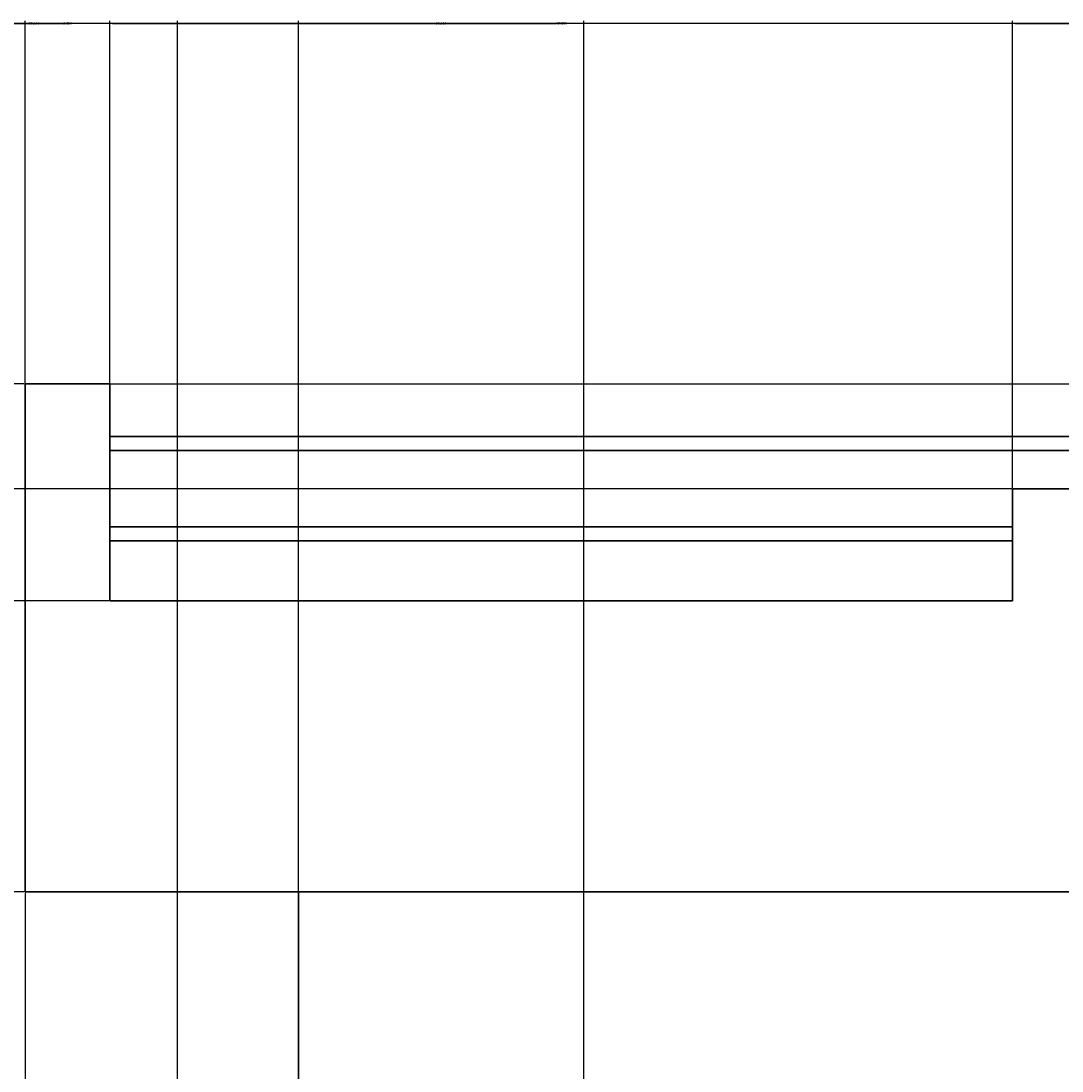
# Model space of a CAD drawing. Units: inches. Extents: x 93 to 565, y 123 to 656.
# Tile 17 of 18: x 418 to 491, y 582 to 656. Entities that reach past the tile are written whole.
import ezdxf

# ---------------------------------------------------------------- set-up
doc = ezdxf.new("R2010")
doc.units = ezdxf.units.IN
doc.header["$MEASUREMENT"] = 0
doc.layers.add('A-ANNO-DIMS', color=2, linetype='Continuous', lineweight=18)
doc.layers.add('A-ELEV', color=7, linetype='Continuous', lineweight=35)
doc.styles.get("Standard").update_dxf_attribs({"font": 'arial.ttf'})
doc.dimstyles.get("Standard").update_dxf_attribs({"dimtxt": 0.18, "dimasz": 0.18, "dimexe": 0.18, "dimexo": 0.0625, "dimgap": 0.09, "dimtad": 0, "dimtih": 1, "dimtoh": 1, "dimdec": 4, "dimzin": 0, "dimdsep": 46, "dimtxsty": 'Standard', "dimcen": 0.09, "dimadec": 0, "dimazin": 0, "dimtfac": 1, "dimtdec": 4, "dimtofl": 0, "dimtmove": 0, "dimatfit": 3, "dimfxl": 1, "dimtolj": 1, "dimtzin": 0, "dimarcsym": 0})

# ---------------------------------------------------------------- blocks, each defined once
blk = doc.blocks.new('*D26')
at = {"layer": 'A-ANNO-DIMS', "color": 0, "lineweight": -2, "transparency": 16777216}
for p, q in [((119.079, 519.162), (119.079, 656.135)), ((119.259, 655.955), (328.787, 655.955)), ((538.899, 655.955), (329.372, 655.955)), ((539.079, 630.467), (539.079, 656.135))]:
    blk.add_line(p, q, dxfattribs=at)
at = {"layer": 'A-ANNO-DIMS', "color": 0, "transparency": 16777216}
for points in [[(119.259, 655.985), (119.259, 655.925), (119.079, 655.955)], [(538.899, 655.985), (538.899, 655.925), (539.079, 655.955)]]:
    blk.add_solid(points, dxfattribs=at)
at = {"layer": 'Defpoints', "color": 0, "transparency": 16777216}
for p in [(539.079, 655.955), (539.079, 630.405), (119.079, 519.1)]:
    blk.add_point(p, dxfattribs=at)
at = {"layer": 'A-ANNO-DIMS', "color": 0, "transparency": 16777216, "insert": (329.079, 655.955), "char_height": 0.18, "attachment_point": 5}
blk.add_mtext('\\A1;420', dxfattribs=at)
blk = doc.blocks.new('*D29')
at = {"layer": 'A-ANNO-DIMS', "color": 0, "lineweight": -2, "transparency": 16777216}
for p, q in [((437.189, 594.342), (437.189, 134.002)), ((295.687, 183.67), (295.687, 134.002)), ((295.867, 134.182), (366.052, 134.182)), ((437.009, 134.182), (366.824, 134.182))]:
    blk.add_line(p, q, dxfattribs=at)
at = {"layer": 'A-ANNO-DIMS', "color": 0, "transparency": 16777216}
for points in [[(295.867, 134.212), (295.867, 134.152), (295.687, 134.182)], [(437.009, 134.212), (437.009, 134.152), (437.189, 134.182)]]:
    blk.add_solid(points, dxfattribs=at)
at = {"layer": 'Defpoints', "color": 0, "transparency": 16777216}
for p in [(437.189, 594.405), (295.687, 183.732), (437.189, 134.182)]:
    blk.add_point(p, dxfattribs=at)
at = {"layer": 'A-ANNO-DIMS', "color": 0, "transparency": 16777216, "insert": (366.438, 134.182), "char_height": 0.18, "attachment_point": 5}
blk.add_mtext('\\A1;141.5', dxfattribs=at)
blk = doc.blocks.new('*D30')
at = {"layer": 'A-ANNO-DIMS', "color": 0, "lineweight": -2, "transparency": 16777216}
for p, q in [((437.189, 594.342), (437.189, 134.002)), ((539.079, 159.67), (539.079, 134.002)), ((437.369, 134.182), (487.749, 134.182)), ((538.899, 134.182), (488.519, 134.182))]:
    blk.add_line(p, q, dxfattribs=at)
at = {"layer": 'A-ANNO-DIMS', "color": 0, "transparency": 16777216}
for points in [[(437.369, 134.212), (437.369, 134.152), (437.189, 134.182)], [(538.899, 134.212), (538.899, 134.152), (539.079, 134.182)]]:
    blk.add_solid(points, dxfattribs=at)
at = {"layer": 'Defpoints', "color": 0, "transparency": 16777216}
for p in [(437.189, 594.405), (539.079, 159.732), (539.079, 134.182)]:
    blk.add_point(p, dxfattribs=at)
at = {"layer": 'A-ANNO-DIMS', "color": 0, "transparency": 16777216, "insert": (488.134, 134.182), "char_height": 0.18, "attachment_point": 5}
blk.add_mtext('\\A1;101.9', dxfattribs=at)
blk = doc.blocks.new('*D31')
at = {"layer": 'A-ANNO-DIMS', "color": 0, "lineweight": -2, "transparency": 16777216}
for p, q in [((417.872, 630.405), (564.809, 630.405)), ((564.629, 630.225), (564.629, 395.25)), ((564.629, 159.912), (564.629, 394.887)), ((119.142, 159.732), (564.809, 159.732))]:
    blk.add_line(p, q, dxfattribs=at)
at = {"layer": 'A-ANNO-DIMS', "color": 0, "transparency": 16777216}
for points in [[(564.599, 630.225), (564.659, 630.225), (564.629, 630.405)], [(564.599, 159.912), (564.659, 159.912), (564.629, 159.732)]]:
    blk.add_solid(points, dxfattribs=at)
at = {"layer": 'Defpoints', "color": 0, "transparency": 16777216}
for p in [(417.81, 630.405), (564.629, 630.405), (119.079, 159.732)]:
    blk.add_point(p, dxfattribs=at)
at = {"layer": 'A-ANNO-DIMS', "color": 0, "transparency": 16777216, "insert": (564.629, 395.069), "char_height": 0.18, "attachment_point": 5}
blk.add_mtext('\\A1;470.7', dxfattribs=at)
blk = doc.blocks.new('*D36')
at = {"layer": 'A-ANNO-DIMS', "color": 0, "lineweight": -2, "transparency": 16777216}
for p, q in [((417.747, 594.405), (93.349, 594.405)), ((93.529, 594.225), (93.529, 556.934)), ((93.529, 519.28), (93.529, 556.57)), ((119.017, 519.1), (93.349, 519.1))]:
    blk.add_line(p, q, dxfattribs=at)
at = {"layer": 'A-ANNO-DIMS', "color": 0, "transparency": 16777216}
for points in [[(93.499, 594.225), (93.559, 594.225), (93.529, 594.405)], [(93.499, 519.28), (93.559, 519.28), (93.529, 519.1)]]:
    blk.add_solid(points, dxfattribs=at)
at = {"layer": 'Defpoints', "color": 0, "transparency": 16777216}
for p in [(93.529, 594.405), (417.81, 594.405), (119.079, 519.1)]:
    blk.add_point(p, dxfattribs=at)
at = {"layer": 'A-ANNO-DIMS', "color": 0, "transparency": 16777216, "insert": (93.529, 556.752), "char_height": 0.18, "attachment_point": 5}
blk.add_mtext('\\A1;75.3', dxfattribs=at)
blk = doc.blocks.new('*D69')
at = {"layer": 'A-ANNO-DIMS', "color": 0, "lineweight": -2, "transparency": 16777216}
for p, q in [((355.46, 420.63), (355.46, 656.135)), ((355.64, 655.955), (391.645, 655.955)), ((428.436, 655.955), (392.431, 655.955)), ((428.616, 420.63), (428.616, 656.135))]:
    blk.add_line(p, q, dxfattribs=at)
at = {"layer": 'A-ANNO-DIMS', "color": 0, "transparency": 16777216}
for points in [[(355.64, 655.985), (355.64, 655.925), (355.46, 655.955)], [(428.436, 655.985), (428.436, 655.925), (428.616, 655.955)]]:
    blk.add_solid(points, dxfattribs=at)
at = {"layer": 'Defpoints', "color": 0, "transparency": 16777216}
for p in [(428.616, 655.955), (355.46, 420.567), (428.616, 420.567)]:
    blk.add_point(p, dxfattribs=at)
at = {"layer": 'A-ANNO-DIMS', "color": 0, "transparency": 16777216, "insert": (392.038, 655.955), "char_height": 0.18, "attachment_point": 5}
blk.add_mtext('\\A1;73.16', dxfattribs=at)
blk = doc.blocks.new('*D76')
at = {"layer": 'A-ANNO-DIMS', "color": 0, "lineweight": -2, "transparency": 16777216}
for p, q in [((399.695, 507.892), (399.695, 656.135)), ((399.875, 655.955), (417.978, 655.955)), ((437.009, 655.955), (418.905, 655.955)), ((437.189, 507.795), (437.189, 656.135))]:
    blk.add_line(p, q, dxfattribs=at)
at = {"layer": 'A-ANNO-DIMS', "color": 0, "transparency": 16777216}
for points in [[(399.875, 655.985), (399.875, 655.925), (399.695, 655.955)], [(437.009, 655.985), (437.009, 655.925), (437.189, 655.955)]]:
    blk.add_solid(points, dxfattribs=at)
at = {"layer": 'Defpoints', "color": 0, "transparency": 16777216}
for p in [(437.189, 655.955), (399.695, 507.83), (437.189, 507.732)]:
    blk.add_point(p, dxfattribs=at)
at = {"layer": 'A-ANNO-DIMS', "color": 0, "transparency": 16777216, "insert": (418.442, 655.955), "char_height": 0.18, "attachment_point": 5}
blk.add_mtext('\\A1;37.494', dxfattribs=at)
blk = doc.blocks.new('*D82')
at = {"layer": 'A-ANNO-DIMS', "color": 0, "lineweight": -2, "transparency": 16777216}
for p, q in [((437.189, 447.795), (437.189, 656.135)), ((437.369, 655.955), (446.825, 655.955)), ((457.213, 655.955), (447.757, 655.955)), ((457.393, 378.4), (457.393, 656.135))]:
    blk.add_line(p, q, dxfattribs=at)
at = {"layer": 'A-ANNO-DIMS', "color": 0, "transparency": 16777216}
for points in [[(437.369, 655.985), (437.369, 655.925), (437.189, 655.955)], [(457.213, 655.985), (457.213, 655.925), (457.393, 655.955)]]:
    blk.add_solid(points, dxfattribs=at)
at = {"layer": 'Defpoints', "color": 0, "transparency": 16777216}
for p in [(457.393, 655.955), (437.189, 447.732), (457.393, 378.337)]:
    blk.add_point(p, dxfattribs=at)
at = {"layer": 'A-ANNO-DIMS', "color": 0, "transparency": 16777216, "insert": (447.291, 655.955), "char_height": 0.18, "attachment_point": 5}
blk.add_mtext('\\A1;20.205', dxfattribs=at)
blk = doc.blocks.new('*D86')
at = {"layer": 'A-ANNO-DIMS', "color": 0, "lineweight": -2, "transparency": 16777216}
for p, q in [((417.81, 630.467), (417.81, 656.135)), ((417.99, 655.955), (420.66, 655.955)), ((423.63, 655.955), (420.959, 655.955)), ((423.81, 630.467), (423.81, 656.135))]:
    blk.add_line(p, q, dxfattribs=at)
at = {"layer": 'A-ANNO-DIMS', "color": 0, "transparency": 16777216}
for points in [[(417.99, 655.985), (417.99, 655.925), (417.81, 655.955)], [(423.63, 655.985), (423.63, 655.925), (423.81, 655.955)]]:
    blk.add_solid(points, dxfattribs=at)
at = {"layer": 'Defpoints', "color": 0, "transparency": 16777216}
for p in [(423.81, 655.955), (417.81, 630.405), (423.81, 630.405)]:
    blk.add_point(p, dxfattribs=at)
at = {"layer": 'A-ANNO-DIMS', "color": 0, "transparency": 16777216, "insert": (420.81, 655.955), "char_height": 0.18, "attachment_point": 5}
blk.add_mtext('\\A1;6', dxfattribs=at)
blk = doc.blocks.new('*D87')
at = {"layer": 'A-ANNO-DIMS', "color": 0, "lineweight": -2, "transparency": 16777216}
for p, q in [((423.81, 630.467), (423.81, 656.135)), ((423.99, 655.955), (455.408, 655.955)), ((487.615, 655.955), (456.197, 655.955)), ((487.795, 623.034), (487.795, 656.135))]:
    blk.add_line(p, q, dxfattribs=at)
at = {"layer": 'A-ANNO-DIMS', "color": 0, "transparency": 16777216}
for points in [[(423.99, 655.985), (423.99, 655.925), (423.81, 655.955)], [(487.615, 655.985), (487.615, 655.925), (487.795, 655.955)]]:
    blk.add_solid(points, dxfattribs=at)
at = {"layer": 'Defpoints', "color": 0, "transparency": 16777216}
for p in [(487.795, 655.955), (423.81, 630.405), (487.795, 622.971)]:
    blk.add_point(p, dxfattribs=at)
at = {"layer": 'A-ANNO-DIMS', "color": 0, "transparency": 16777216, "insert": (455.802, 655.955), "char_height": 0.18, "attachment_point": 5}
blk.add_mtext('\\A1;63.99', dxfattribs=at)
blk = doc.blocks.new('*D88')
at = {"layer": 'A-ANNO-DIMS', "color": 0, "lineweight": -2, "transparency": 16777216}
for p, q in [((487.795, 623.034), (487.795, 656.135)), ((487.975, 655.955), (500.917, 655.955)), ((514.789, 655.955), (501.847, 655.955)), ((514.969, 630.467), (514.969, 656.135))]:
    blk.add_line(p, q, dxfattribs=at)
at = {"layer": 'A-ANNO-DIMS', "color": 0, "transparency": 16777216}
for points in [[(487.975, 655.985), (487.975, 655.925), (487.795, 655.955)], [(514.789, 655.985), (514.789, 655.925), (514.969, 655.955)]]:
    blk.add_solid(points, dxfattribs=at)
at = {"layer": 'Defpoints', "color": 0, "transparency": 16777216}
for p in [(514.969, 655.955), (514.969, 630.405), (487.795, 622.971)]:
    blk.add_point(p, dxfattribs=at)
at = {"layer": 'A-ANNO-DIMS', "color": 0, "transparency": 16777216, "insert": (501.382, 655.955), "char_height": 0.18, "attachment_point": 5}
blk.add_mtext('\\A1;27.174', dxfattribs=at)
blk = doc.blocks.new('*D90')
at = {"layer": 'A-ANNO-DIMS', "color": 0, "lineweight": -2, "transparency": 16777216}
for p, q in [((417.81, 594.342), (417.81, 134.002)), ((437.189, 594.342), (437.189, 134.002)), ((417.99, 134.182), (427.114, 134.182)), ((437.009, 134.182), (427.885, 134.182))]:
    blk.add_line(p, q, dxfattribs=at)
at = {"layer": 'A-ANNO-DIMS', "color": 0, "transparency": 16777216}
for points in [[(417.99, 134.212), (417.99, 134.152), (417.81, 134.182)], [(437.009, 134.212), (437.009, 134.152), (437.189, 134.182)]]:
    blk.add_solid(points, dxfattribs=at)
at = {"layer": 'Defpoints', "color": 0, "transparency": 16777216}
for p in [(417.81, 594.405), (437.189, 594.405), (437.189, 134.182)]:
    blk.add_point(p, dxfattribs=at)
at = {"layer": 'A-ANNO-DIMS', "color": 0, "transparency": 16777216, "insert": (427.499, 134.182), "char_height": 0.18, "attachment_point": 5}
blk.add_mtext('\\A1;19.38', dxfattribs=at)
blk = doc.blocks.new('*D91')
at = {"layer": 'A-ANNO-DIMS', "color": 0, "lineweight": -2, "transparency": 16777216}
for p, q in [((499.729, 599.755), (499.729, 134.002)), ((437.189, 594.342), (437.189, 134.002)), ((437.369, 134.182), (468.065, 134.182)), ((499.549, 134.182), (468.853, 134.182))]:
    blk.add_line(p, q, dxfattribs=at)
at = {"layer": 'A-ANNO-DIMS', "color": 0, "transparency": 16777216}
for points in [[(437.369, 134.212), (437.369, 134.152), (437.189, 134.182)], [(499.549, 134.212), (499.549, 134.152), (499.729, 134.182)]]:
    blk.add_solid(points, dxfattribs=at)
at = {"layer": 'Defpoints', "color": 0, "transparency": 16777216}
for p in [(499.729, 599.817), (437.189, 594.405), (499.729, 134.182)]:
    blk.add_point(p, dxfattribs=at)
at = {"layer": 'A-ANNO-DIMS', "color": 0, "transparency": 16777216, "insert": (468.459, 134.182), "char_height": 0.18, "attachment_point": 5}
blk.add_mtext('\\A1;62.54', dxfattribs=at)
blk = doc.blocks.new('*D94')
at = {"layer": 'A-ANNO-DIMS', "color": 0, "lineweight": -2, "transparency": 16777216}
for p, q in [((423.747, 615.041), (93.349, 615.041)), ((93.529, 614.861), (93.529, 604.905)), ((93.529, 594.585), (93.529, 604.541)), ((417.747, 594.405), (93.349, 594.405))]:
    blk.add_line(p, q, dxfattribs=at)
at = {"layer": 'A-ANNO-DIMS', "color": 0, "transparency": 16777216}
for points in [[(93.499, 614.861), (93.559, 614.861), (93.529, 615.041)], [(93.499, 594.585), (93.559, 594.585), (93.529, 594.405)]]:
    blk.add_solid(points, dxfattribs=at)
at = {"layer": 'Defpoints', "color": 0, "transparency": 16777216}
for p in [(93.529, 615.041), (423.81, 615.041), (417.81, 594.405)]:
    blk.add_point(p, dxfattribs=at)
at = {"layer": 'A-ANNO-DIMS', "color": 0, "transparency": 16777216, "insert": (93.529, 604.723), "char_height": 0.18, "attachment_point": 5}
blk.add_mtext('\\A1;20.636', dxfattribs=at)
blk = doc.blocks.new('*D95')
at = {"layer": 'A-ANNO-DIMS', "color": 0, "lineweight": -2, "transparency": 16777216}
for p, q in [((487.733, 622.971), (93.349, 622.971)), ((93.529, 622.791), (93.529, 619.188)), ((93.529, 615.221), (93.529, 618.824)), ((423.747, 615.041), (93.349, 615.041))]:
    blk.add_line(p, q, dxfattribs=at)
at = {"layer": 'A-ANNO-DIMS', "color": 0, "transparency": 16777216}
for points in [[(93.499, 622.791), (93.559, 622.791), (93.529, 622.971)], [(93.499, 615.221), (93.559, 615.221), (93.529, 615.041)]]:
    blk.add_solid(points, dxfattribs=at)
at = {"layer": 'Defpoints', "color": 0, "transparency": 16777216}
for p in [(93.529, 622.971), (487.795, 622.971), (423.81, 615.041)]:
    blk.add_point(p, dxfattribs=at)
at = {"layer": 'A-ANNO-DIMS', "color": 0, "transparency": 16777216, "insert": (93.529, 619.006), "char_height": 0.18, "attachment_point": 5}
blk.add_mtext('\\A1;7.93', dxfattribs=at)
blk = doc.blocks.new('*D96')
at = {"layer": 'A-ANNO-DIMS', "color": 0, "lineweight": -2, "transparency": 16777216}
for p, q in [((417.747, 630.405), (93.349, 630.405)), ((93.529, 630.225), (93.529, 626.87)), ((93.529, 623.151), (93.529, 626.506)), ((487.733, 622.971), (93.349, 622.971))]:
    blk.add_line(p, q, dxfattribs=at)
at = {"layer": 'A-ANNO-DIMS', "color": 0, "transparency": 16777216}
for points in [[(93.499, 630.225), (93.559, 630.225), (93.529, 630.405)], [(93.499, 623.151), (93.559, 623.151), (93.529, 622.971)]]:
    blk.add_solid(points, dxfattribs=at)
at = {"layer": 'Defpoints', "color": 0, "transparency": 16777216}
for p in [(93.529, 630.405), (417.81, 630.405), (487.795, 622.971)]:
    blk.add_point(p, dxfattribs=at)
at = {"layer": 'A-ANNO-DIMS', "color": 0, "transparency": 16777216, "insert": (93.529, 626.688), "char_height": 0.18, "attachment_point": 5}
blk.add_mtext('\\A1;7.434', dxfattribs=at)
blk = doc.blocks.new('*D100')
at = {"layer": 'A-ANNO-DIMS', "color": 0, "lineweight": -2, "transparency": 16777216}
for p, q in [((499.792, 599.817), (564.809, 599.817)), ((564.629, 599.637), (564.629, 597.293)), ((564.629, 594.585), (564.629, 596.929)), ((437.251, 594.405), (564.809, 594.405))]:
    blk.add_line(p, q, dxfattribs=at)
at = {"layer": 'A-ANNO-DIMS', "color": 0, "transparency": 16777216}
for points in [[(564.599, 599.637), (564.659, 599.637), (564.629, 599.817)], [(564.599, 594.585), (564.659, 594.585), (564.629, 594.405)]]:
    blk.add_solid(points, dxfattribs=at)
at = {"layer": 'Defpoints', "color": 0, "transparency": 16777216}
for p in [(499.729, 599.817), (437.189, 594.405), (564.629, 594.405)]:
    blk.add_point(p, dxfattribs=at)
at = {"layer": 'A-ANNO-DIMS', "color": 0, "transparency": 16777216, "insert": (564.629, 597.111), "char_height": 0.18, "attachment_point": 5}
blk.add_mtext('\\A1;5.412', dxfattribs=at)
blk = doc.blocks.new('*D105')
at = {"layer": 'A-ANNO-DIMS', "color": 0, "lineweight": -2, "transparency": 16777216}
for p, q in [((119.079, 519.162), (119.079, 656.135)), ((119.259, 655.955), (328.542, 655.955)), ((538.899, 655.955), (329.616, 655.955)), ((539.079, 630.467), (539.079, 656.135))]:
    blk.add_line(p, q, dxfattribs=at)
at = {"layer": 'A-ANNO-DIMS', "color": 0, "transparency": 16777216}
for points in [[(119.259, 655.985), (119.259, 655.925), (119.079, 655.955)], [(538.899, 655.985), (538.899, 655.925), (539.079, 655.955)]]:
    blk.add_solid(points, dxfattribs=at)
at = {"layer": 'Defpoints', "color": 0, "transparency": 16777216}
for p in [(539.079, 655.955), (539.079, 630.405), (119.079, 519.1)]:
    blk.add_point(p, dxfattribs=at)
at = {"layer": 'A-ANNO-DIMS', "color": 0, "transparency": 16777216, "insert": (329.079, 655.955), "char_height": 0.18, "attachment_point": 5}
blk.add_mtext('\\A1;420.000', dxfattribs=at)
blk = doc.blocks.new('*D108')
at = {"layer": 'A-ANNO-DIMS', "color": 0, "lineweight": -2, "transparency": 16777216}
for p, q in [((437.189, 594.342), (437.189, 134.002)), ((295.687, 183.67), (295.687, 134.002)), ((295.867, 134.182), (365.93, 134.182)), ((437.009, 134.182), (366.946, 134.182))]:
    blk.add_line(p, q, dxfattribs=at)
at = {"layer": 'A-ANNO-DIMS', "color": 0, "transparency": 16777216}
for points in [[(295.867, 134.212), (295.867, 134.152), (295.687, 134.182)], [(437.009, 134.212), (437.009, 134.152), (437.189, 134.182)]]:
    blk.add_solid(points, dxfattribs=at)
at = {"layer": 'Defpoints', "color": 0, "transparency": 16777216}
for p in [(437.189, 594.405), (295.687, 183.732), (437.189, 134.182)]:
    blk.add_point(p, dxfattribs=at)
at = {"layer": 'A-ANNO-DIMS', "color": 0, "transparency": 16777216, "insert": (366.438, 134.182), "char_height": 0.18, "attachment_point": 5}
blk.add_mtext('\\A1;141.501', dxfattribs=at)
blk = doc.blocks.new('*D109')
at = {"layer": 'A-ANNO-DIMS', "color": 0, "lineweight": -2, "transparency": 16777216}
for p, q in [((437.189, 594.342), (437.189, 134.002)), ((539.079, 159.67), (539.079, 134.002)), ((437.369, 134.182), (487.626, 134.182)), ((538.899, 134.182), (488.642, 134.182))]:
    blk.add_line(p, q, dxfattribs=at)
at = {"layer": 'A-ANNO-DIMS', "color": 0, "transparency": 16777216}
for points in [[(437.369, 134.212), (437.369, 134.152), (437.189, 134.182)], [(538.899, 134.212), (538.899, 134.152), (539.079, 134.182)]]:
    blk.add_solid(points, dxfattribs=at)
at = {"layer": 'Defpoints', "color": 0, "transparency": 16777216}
for p in [(437.189, 594.405), (539.079, 159.732), (539.079, 134.182)]:
    blk.add_point(p, dxfattribs=at)
at = {"layer": 'A-ANNO-DIMS', "color": 0, "transparency": 16777216, "insert": (488.134, 134.182), "char_height": 0.18, "attachment_point": 5}
blk.add_mtext('\\A1;101.891', dxfattribs=at)
blk = doc.blocks.new('*D110')
at = {"layer": 'A-ANNO-DIMS', "color": 0, "lineweight": -2, "transparency": 16777216}
for p, q in [((417.872, 630.405), (564.809, 630.405)), ((564.629, 630.225), (564.629, 395.25)), ((564.629, 159.912), (564.629, 394.887)), ((119.142, 159.732), (564.809, 159.732))]:
    blk.add_line(p, q, dxfattribs=at)
at = {"layer": 'A-ANNO-DIMS', "color": 0, "transparency": 16777216}
for points in [[(564.599, 630.225), (564.659, 630.225), (564.629, 630.405)], [(564.599, 159.912), (564.659, 159.912), (564.629, 159.732)]]:
    blk.add_solid(points, dxfattribs=at)
at = {"layer": 'Defpoints', "color": 0, "transparency": 16777216}
for p in [(417.81, 630.405), (564.629, 630.405), (119.079, 159.732)]:
    blk.add_point(p, dxfattribs=at)
at = {"layer": 'A-ANNO-DIMS', "color": 0, "transparency": 16777216, "insert": (564.629, 395.069), "char_height": 0.18, "attachment_point": 5}
blk.add_mtext('\\A1;470.673', dxfattribs=at)
blk = doc.blocks.new('*D115')
at = {"layer": 'A-ANNO-DIMS', "color": 0, "lineweight": -2, "transparency": 16777216}
for p, q in [((417.747, 594.405), (93.349, 594.405)), ((93.529, 594.225), (93.529, 556.934)), ((93.529, 519.28), (93.529, 556.57)), ((119.017, 519.1), (93.349, 519.1))]:
    blk.add_line(p, q, dxfattribs=at)
at = {"layer": 'A-ANNO-DIMS', "color": 0, "transparency": 16777216}
for points in [[(93.499, 594.225), (93.559, 594.225), (93.529, 594.405)], [(93.499, 519.28), (93.559, 519.28), (93.529, 519.1)]]:
    blk.add_solid(points, dxfattribs=at)
at = {"layer": 'Defpoints', "color": 0, "transparency": 16777216}
for p in [(93.529, 594.405), (417.81, 594.405), (119.079, 519.1)]:
    blk.add_point(p, dxfattribs=at)
at = {"layer": 'A-ANNO-DIMS', "color": 0, "transparency": 16777216, "insert": (93.529, 556.752), "char_height": 0.18, "attachment_point": 5}
blk.add_mtext('\\A1;75.305', dxfattribs=at)
blk = doc.blocks.new('*D148')
at = {"layer": 'A-ANNO-DIMS', "color": 0, "lineweight": -2, "transparency": 16777216}
for p, q in [((355.46, 420.63), (355.46, 656.135)), ((355.64, 655.955), (391.575, 655.955)), ((428.436, 655.955), (392.501, 655.955)), ((428.616, 420.63), (428.616, 656.135))]:
    blk.add_line(p, q, dxfattribs=at)
at = {"layer": 'A-ANNO-DIMS', "color": 0, "transparency": 16777216}
for points in [[(355.64, 655.985), (355.64, 655.925), (355.46, 655.955)], [(428.436, 655.985), (428.436, 655.925), (428.616, 655.955)]]:
    blk.add_solid(points, dxfattribs=at)
at = {"layer": 'Defpoints', "color": 0, "transparency": 16777216}
for p in [(428.616, 655.955), (355.46, 420.567), (428.616, 420.567)]:
    blk.add_point(p, dxfattribs=at)
at = {"layer": 'A-ANNO-DIMS', "color": 0, "transparency": 16777216, "insert": (392.038, 655.955), "char_height": 0.18, "attachment_point": 5}
blk.add_mtext('\\A1;73.156', dxfattribs=at)
blk = doc.blocks.new('*D155')
at = {"layer": 'A-ANNO-DIMS', "color": 0, "lineweight": -2, "transparency": 16777216}
for p, q in [((399.695, 507.892), (399.695, 656.135)), ((399.875, 655.955), (417.978, 655.955)), ((437.009, 655.955), (418.905, 655.955)), ((437.189, 507.795), (437.189, 656.135))]:
    blk.add_line(p, q, dxfattribs=at)
at = {"layer": 'A-ANNO-DIMS', "color": 0, "transparency": 16777216}
for points in [[(399.875, 655.985), (399.875, 655.925), (399.695, 655.955)], [(437.009, 655.985), (437.009, 655.925), (437.189, 655.955)]]:
    blk.add_solid(points, dxfattribs=at)
at = {"layer": 'Defpoints', "color": 0, "transparency": 16777216}
for p in [(437.189, 655.955), (399.695, 507.83), (437.189, 507.732)]:
    blk.add_point(p, dxfattribs=at)
at = {"layer": 'A-ANNO-DIMS', "color": 0, "transparency": 16777216, "insert": (418.442, 655.955), "char_height": 0.18, "attachment_point": 5}
blk.add_mtext('\\A1;37.494', dxfattribs=at)
blk = doc.blocks.new('*D161')
at = {"layer": 'A-ANNO-DIMS', "color": 0, "lineweight": -2, "transparency": 16777216}
for p, q in [((437.189, 447.795), (437.189, 656.135)), ((437.369, 655.955), (446.825, 655.955)), ((457.213, 655.955), (447.757, 655.955)), ((457.393, 378.4), (457.393, 656.135))]:
    blk.add_line(p, q, dxfattribs=at)
at = {"layer": 'A-ANNO-DIMS', "color": 0, "transparency": 16777216}
for points in [[(437.369, 655.985), (437.369, 655.925), (437.189, 655.955)], [(457.213, 655.985), (457.213, 655.925), (457.393, 655.955)]]:
    blk.add_solid(points, dxfattribs=at)
at = {"layer": 'Defpoints', "color": 0, "transparency": 16777216}
for p in [(457.393, 655.955), (437.189, 447.732), (457.393, 378.337)]:
    blk.add_point(p, dxfattribs=at)
at = {"layer": 'A-ANNO-DIMS', "color": 0, "transparency": 16777216, "insert": (447.291, 655.955), "char_height": 0.18, "attachment_point": 5}
blk.add_mtext('\\A1;20.205', dxfattribs=at)
blk = doc.blocks.new('*D165')
at = {"layer": 'A-ANNO-DIMS', "color": 0, "lineweight": -2, "transparency": 16777216}
for p, q in [((417.81, 630.467), (417.81, 656.135)), ((417.99, 655.955), (420.416, 655.955)), ((423.63, 655.955), (421.204, 655.955)), ((423.81, 630.467), (423.81, 656.135))]:
    blk.add_line(p, q, dxfattribs=at)
at = {"layer": 'A-ANNO-DIMS', "color": 0, "transparency": 16777216}
for points in [[(417.99, 655.985), (417.99, 655.925), (417.81, 655.955)], [(423.63, 655.985), (423.63, 655.925), (423.81, 655.955)]]:
    blk.add_solid(points, dxfattribs=at)
at = {"layer": 'Defpoints', "color": 0, "transparency": 16777216}
for p in [(423.81, 655.955), (417.81, 630.405), (423.81, 630.405)]:
    blk.add_point(p, dxfattribs=at)
at = {"layer": 'A-ANNO-DIMS', "color": 0, "transparency": 16777216, "insert": (420.81, 655.955), "char_height": 0.18, "attachment_point": 5}
blk.add_mtext('\\A1;6.000', dxfattribs=at)
blk = doc.blocks.new('*D166')
at = {"layer": 'A-ANNO-DIMS', "color": 0, "lineweight": -2, "transparency": 16777216}
for p, q in [((423.81, 630.467), (423.81, 656.135)), ((423.99, 655.955), (455.338, 655.955)), ((487.615, 655.955), (456.267, 655.955)), ((487.795, 623.034), (487.795, 656.135))]:
    blk.add_line(p, q, dxfattribs=at)
at = {"layer": 'A-ANNO-DIMS', "color": 0, "transparency": 16777216}
for points in [[(423.99, 655.985), (423.99, 655.925), (423.81, 655.955)], [(487.615, 655.985), (487.615, 655.925), (487.795, 655.955)]]:
    blk.add_solid(points, dxfattribs=at)
at = {"layer": 'Defpoints', "color": 0, "transparency": 16777216}
for p in [(487.795, 655.955), (423.81, 630.405), (487.795, 622.971)]:
    blk.add_point(p, dxfattribs=at)
at = {"layer": 'A-ANNO-DIMS', "color": 0, "transparency": 16777216, "insert": (455.802, 655.955), "char_height": 0.18, "attachment_point": 5}
blk.add_mtext('\\A1;63.986', dxfattribs=at)
blk = doc.blocks.new('*D167')
at = {"layer": 'A-ANNO-DIMS', "color": 0, "lineweight": -2, "transparency": 16777216}
for p, q in [((487.795, 623.034), (487.795, 656.135)), ((487.975, 655.955), (500.917, 655.955)), ((514.789, 655.955), (501.847, 655.955)), ((514.969, 630.467), (514.969, 656.135))]:
    blk.add_line(p, q, dxfattribs=at)
at = {"layer": 'A-ANNO-DIMS', "color": 0, "transparency": 16777216}
for points in [[(487.975, 655.985), (487.975, 655.925), (487.795, 655.955)], [(514.789, 655.985), (514.789, 655.925), (514.969, 655.955)]]:
    blk.add_solid(points, dxfattribs=at)
at = {"layer": 'Defpoints', "color": 0, "transparency": 16777216}
for p in [(514.969, 655.955), (514.969, 630.405), (487.795, 622.971)]:
    blk.add_point(p, dxfattribs=at)
at = {"layer": 'A-ANNO-DIMS', "color": 0, "transparency": 16777216, "insert": (501.382, 655.955), "char_height": 0.18, "attachment_point": 5}
blk.add_mtext('\\A1;27.174', dxfattribs=at)
blk = doc.blocks.new('*D169')
at = {"layer": 'A-ANNO-DIMS', "color": 0, "lineweight": -2, "transparency": 16777216}
for p, q in [((417.81, 594.342), (417.81, 134.002)), ((437.189, 594.342), (437.189, 134.002)), ((417.99, 134.182), (427.044, 134.182)), ((437.009, 134.182), (427.954, 134.182))]:
    blk.add_line(p, q, dxfattribs=at)
at = {"layer": 'A-ANNO-DIMS', "color": 0, "transparency": 16777216}
for points in [[(417.99, 134.212), (417.99, 134.152), (417.81, 134.182)], [(437.009, 134.212), (437.009, 134.152), (437.189, 134.182)]]:
    blk.add_solid(points, dxfattribs=at)
at = {"layer": 'Defpoints', "color": 0, "transparency": 16777216}
for p in [(417.81, 594.405), (437.189, 594.405), (437.189, 134.182)]:
    blk.add_point(p, dxfattribs=at)
at = {"layer": 'A-ANNO-DIMS', "color": 0, "transparency": 16777216, "insert": (427.499, 134.182), "char_height": 0.18, "attachment_point": 5}
blk.add_mtext('\\A1;19.379', dxfattribs=at)
blk = doc.blocks.new('*D170')
at = {"layer": 'A-ANNO-DIMS', "color": 0, "lineweight": -2, "transparency": 16777216}
for p, q in [((499.729, 599.755), (499.729, 134.002)), ((437.189, 594.342), (437.189, 134.002)), ((437.369, 134.182), (468.012, 134.182)), ((499.549, 134.182), (468.906, 134.182))]:
    blk.add_line(p, q, dxfattribs=at)
at = {"layer": 'A-ANNO-DIMS', "color": 0, "transparency": 16777216}
for points in [[(437.369, 134.212), (437.369, 134.152), (437.189, 134.182)], [(499.549, 134.212), (499.549, 134.152), (499.729, 134.182)]]:
    blk.add_solid(points, dxfattribs=at)
at = {"layer": 'Defpoints', "color": 0, "transparency": 16777216}
for p in [(499.729, 599.817), (437.189, 594.405), (499.729, 134.182)]:
    blk.add_point(p, dxfattribs=at)
at = {"layer": 'A-ANNO-DIMS', "color": 0, "transparency": 16777216, "insert": (468.459, 134.182), "char_height": 0.18, "attachment_point": 5}
blk.add_mtext('\\A1;62.541', dxfattribs=at)
blk = doc.blocks.new('*D173')
at = {"layer": 'A-ANNO-DIMS', "color": 0, "lineweight": -2, "transparency": 16777216}
for p, q in [((423.747, 615.041), (93.349, 615.041)), ((93.529, 614.861), (93.529, 604.905)), ((93.529, 594.585), (93.529, 604.541)), ((417.747, 594.405), (93.349, 594.405))]:
    blk.add_line(p, q, dxfattribs=at)
at = {"layer": 'A-ANNO-DIMS', "color": 0, "transparency": 16777216}
for points in [[(93.499, 614.861), (93.559, 614.861), (93.529, 615.041)], [(93.499, 594.585), (93.559, 594.585), (93.529, 594.405)]]:
    blk.add_solid(points, dxfattribs=at)
at = {"layer": 'Defpoints', "color": 0, "transparency": 16777216}
for p in [(93.529, 615.041), (423.81, 615.041), (417.81, 594.405)]:
    blk.add_point(p, dxfattribs=at)
at = {"layer": 'A-ANNO-DIMS', "color": 0, "transparency": 16777216, "insert": (93.529, 604.723), "char_height": 0.18, "attachment_point": 5}
blk.add_mtext('\\A1;20.636', dxfattribs=at)
blk = doc.blocks.new('*D174')
at = {"layer": 'A-ANNO-DIMS', "color": 0, "lineweight": -2, "transparency": 16777216}
for p, q in [((487.733, 622.971), (93.349, 622.971)), ((93.529, 622.791), (93.529, 619.188)), ((93.529, 615.221), (93.529, 618.824)), ((423.747, 615.041), (93.349, 615.041))]:
    blk.add_line(p, q, dxfattribs=at)
at = {"layer": 'A-ANNO-DIMS', "color": 0, "transparency": 16777216}
for points in [[(93.499, 622.791), (93.559, 622.791), (93.529, 622.971)], [(93.499, 615.221), (93.559, 615.221), (93.529, 615.041)]]:
    blk.add_solid(points, dxfattribs=at)
at = {"layer": 'Defpoints', "color": 0, "transparency": 16777216}
for p in [(93.529, 622.971), (487.795, 622.971), (423.81, 615.041)]:
    blk.add_point(p, dxfattribs=at)
at = {"layer": 'A-ANNO-DIMS', "color": 0, "transparency": 16777216, "insert": (93.529, 619.006), "char_height": 0.18, "attachment_point": 5}
blk.add_mtext('\\A1;7.930', dxfattribs=at)
blk = doc.blocks.new('*D175')
at = {"layer": 'A-ANNO-DIMS', "color": 0, "lineweight": -2, "transparency": 16777216}
for p, q in [((417.747, 630.405), (93.349, 630.405)), ((93.529, 630.225), (93.529, 626.87)), ((93.529, 623.151), (93.529, 626.506)), ((487.733, 622.971), (93.349, 622.971))]:
    blk.add_line(p, q, dxfattribs=at)
at = {"layer": 'A-ANNO-DIMS', "color": 0, "transparency": 16777216}
for points in [[(93.499, 630.225), (93.559, 630.225), (93.529, 630.405)], [(93.499, 623.151), (93.559, 623.151), (93.529, 622.971)]]:
    blk.add_solid(points, dxfattribs=at)
at = {"layer": 'Defpoints', "color": 0, "transparency": 16777216}
for p in [(93.529, 630.405), (417.81, 630.405), (487.795, 622.971)]:
    blk.add_point(p, dxfattribs=at)
at = {"layer": 'A-ANNO-DIMS', "color": 0, "transparency": 16777216, "insert": (93.529, 626.688), "char_height": 0.18, "attachment_point": 5}
blk.add_mtext('\\A1;7.434', dxfattribs=at)
blk = doc.blocks.new('*D179')
at = {"layer": 'A-ANNO-DIMS', "color": 0, "lineweight": -2, "transparency": 16777216}
for p, q in [((499.792, 599.817), (564.809, 599.817)), ((564.629, 599.637), (564.629, 597.293)), ((564.629, 594.585), (564.629, 596.929)), ((437.251, 594.405), (564.809, 594.405))]:
    blk.add_line(p, q, dxfattribs=at)
at = {"layer": 'A-ANNO-DIMS', "color": 0, "transparency": 16777216}
for points in [[(564.599, 599.637), (564.659, 599.637), (564.629, 599.817)], [(564.599, 594.585), (564.659, 594.585), (564.629, 594.405)]]:
    blk.add_solid(points, dxfattribs=at)
at = {"layer": 'Defpoints', "color": 0, "transparency": 16777216}
for p in [(499.729, 599.817), (437.189, 594.405), (564.629, 594.405)]:
    blk.add_point(p, dxfattribs=at)
at = {"layer": 'A-ANNO-DIMS', "color": 0, "transparency": 16777216, "insert": (564.629, 597.111), "char_height": 0.18, "attachment_point": 5}
blk.add_mtext('\\A1;5.412', dxfattribs=at)

msp = doc.modelspace()

# ---------------------------------------------------------------- linework, layer by layer
at = {"layer": 'A-ELEV'}
for p, q in [((417.8097, 630.4048), (423.8097, 630.4048)), ((417.8097, 594.4048), (417.8097, 630.4048)), ((417.8097, 630.4048), (423.8097, 630.4048)), ((423.8097, 630.4048), (423.8097, 615.0406)), ((514.9688, 626.6879), (423.8097, 626.6879)), ((514.9688, 625.6879), (423.8097, 625.6879)), ((514.9688, 622.9711), (487.7953, 622.9711)), ((487.7953, 622.9711), (487.7953, 617.5945)), ((487.7953, 620.2828), (423.8097, 620.2828)), ((487.7953, 619.2828), (423.8097, 619.2828)), ((487.7953, 617.5945), (487.7953, 615.0406)), ((487.7953, 615.0406), (423.8097, 615.0406)), ((437.1885, 594.4048), (417.8097, 594.4048)), ((539.0794, 594.4048), (437.1885, 594.4048)), ((437.1885, 594.4048), (437.1885, 507.7323))]:
    msp.add_line(p, q, dxfattribs=at)

# ---------------------------------------------------------------- dimensions: what is measured, and where the dimension line sits
at = {"layer": 'A-ANNO-DIMS'}
for base, p1, p2, override, picture, middle in [((539.0794, 655.9548), (119.0794, 519.0999), (539.0794, 630.4048), {"dimdec": 0, "dimlfac": 1, "dimrnd": 0, "dimzin": 0, "dimdsep": 46, "dimlunit": 2}, '*D26', (329.0794, 655.9548)), ((539.0794, 655.9548), (119.0794, 519.0999), (539.0794, 630.4048), {"dimdec": 3, "dimlfac": 1, "dimrnd": 0, "dimzin": 0, "dimdsep": 46, "dimlunit": 2}, '*D105', (329.0794, 655.9548)), ((428.6158, 655.9548), (355.4603, 420.5674), (428.6158, 420.5674), {"dimdec": 2, "dimlfac": 1, "dimrnd": 0, "dimzin": 0, "dimdsep": 46, "dimlunit": 2}, '*D69', (392.038, 655.9548)), ((428.615792, 655.954775), (355.460288, 420.567351), (428.615792, 420.567351), {"dimdec": 3, "dimlfac": 1, "dimrnd": 0, "dimzin": 0, "dimdsep": 46, "dimlunit": 2}, '*D148', (392.03804, 655.954775)), ((437.1885, 655.9548), (399.6946, 507.8299), (437.1885, 507.7323), {"dimdec": 3, "dimlfac": 1, "dimrnd": 0, "dimzin": 0, "dimdsep": 46, "dimlunit": 2}, '*D76', (418.4415, 655.9548)), ((437.1885, 655.9548), (399.6946, 507.8299), (437.1885, 507.7323), {"dimdec": 3, "dimlfac": 1, "dimrnd": 0, "dimzin": 0, "dimdsep": 46, "dimlunit": 2}, '*D155', (418.4415, 655.9548)), ((423.8097, 655.9548), (417.8097, 630.4048), (423.8097, 630.4048), {"dimdec": 0, "dimlfac": 1, "dimrnd": 0, "dimzin": 0, "dimdsep": 46, "dimlunit": 2}, '*D86', (420.8097, 655.9548)), ((423.8097, 655.9548), (417.8097, 630.4048), (423.8097, 630.4048), {"dimdec": 3, "dimlfac": 1, "dimrnd": 0, "dimzin": 0, "dimdsep": 46, "dimlunit": 2}, '*D165', (420.8097, 655.9548)), ((487.7953, 655.9548), (423.8097, 630.4048), (487.7953, 622.9711), {"dimdec": 2, "dimlfac": 1, "dimrnd": 0, "dimzin": 0, "dimdsep": 46, "dimlunit": 2}, '*D87', (455.8025, 655.9548)), ((487.7953, 655.9548), (423.8097, 630.4048), (487.7953, 622.9711), {"dimdec": 3, "dimlfac": 1, "dimrnd": 0, "dimzin": 0, "dimdsep": 46, "dimlunit": 2}, '*D166', (455.8025, 655.9548)), ((457.3933, 655.9548), (437.1885, 447.7323), (457.3933, 378.3372), {"dimdec": 3, "dimlfac": 1, "dimrnd": 0, "dimzin": 0, "dimdsep": 46, "dimlunit": 2}, '*D82', (447.2909, 655.9548)), ((457.3933, 655.9548), (437.1885, 447.7323), (457.3933, 378.3372), {"dimdec": 3, "dimlfac": 1, "dimrnd": 0, "dimzin": 0, "dimdsep": 46, "dimlunit": 2}, '*D161', (447.2909, 655.9548)), ((514.96884, 655.95478), (487.79526, 622.97108), (514.96884, 630.40477), {"dimdec": 3, "dimlfac": 1, "dimrnd": 0, "dimzin": 0, "dimdsep": 46, "dimlunit": 2}, '*D88', (501.38205, 655.95478)), ((514.96884, 655.95478), (487.79526, 622.97108), (514.96884, 630.40477), {"dimdec": 3, "dimlfac": 1, "dimrnd": 0, "dimzin": 0, "dimdsep": 46, "dimlunit": 2}, '*D167', (501.38205, 655.95478)), ((499.7291, 134.1823), (437.1885, 594.4048), (499.7291, 599.8171), {"dimdec": 2, "dimlfac": 1, "dimrnd": 0, "dimzin": 0, "dimdsep": 46, "dimlunit": 2}, '*D91', (468.4588, 134.1823)), ((499.7291, 134.1823), (437.1885, 594.4048), (499.7291, 599.8171), {"dimdec": 3, "dimlfac": 1, "dimrnd": 0, "dimzin": 0, "dimdsep": 46, "dimlunit": 2}, '*D170', (468.4588, 134.1823)), ((437.1885, 134.1823), (295.6874, 183.7323), (437.1885, 594.4048), {"dimdec": 1, "dimlfac": 1, "dimrnd": 0, "dimzin": 0, "dimdsep": 46, "dimlunit": 2}, '*D29', (366.438, 134.1823)), ((437.1885, 134.1823), (295.6874, 183.7323), (437.1885, 594.4048), {"dimdec": 3, "dimlfac": 1, "dimrnd": 0, "dimzin": 0, "dimdsep": 46, "dimlunit": 2}, '*D108', (366.438, 134.1823)), ((437.1885, 134.1823), (417.8097, 594.4048), (437.1885, 594.4048), {"dimdec": 2, "dimlfac": 1, "dimrnd": 0, "dimzin": 0, "dimdsep": 46, "dimlunit": 2}, '*D90', (427.4991, 134.1823)), ((437.1885, 134.1823), (417.8097, 594.4048), (437.1885, 594.4048), {"dimdec": 3, "dimlfac": 1, "dimrnd": 0, "dimzin": 0, "dimdsep": 46, "dimlunit": 2}, '*D169', (427.4991, 134.1823)), ((539.0794, 134.1823), (437.1885, 594.4048), (539.0794, 159.7323), {"dimdec": 1, "dimlfac": 1, "dimrnd": 0, "dimzin": 0, "dimdsep": 46, "dimlunit": 2}, '*D30', (488.1339, 134.1823)), ((539.0794, 134.1823), (437.1885, 594.4048), (539.0794, 159.7323), {"dimdec": 3, "dimlfac": 1, "dimrnd": 0, "dimzin": 0, "dimdsep": 46, "dimlunit": 2}, '*D109', (488.1339, 134.1823))]:
    dim = msp.add_linear_dim(base=base, p1=p1, p2=p2, dimstyle='Standard', override=override, dxfattribs=at)
    dim.commit()
    dim.dimension.update_dxf_attribs({"geometry": picture, "text_midpoint": middle})
for base, p1, p2, override, picture, middle in [((93.5294, 630.4048), (487.7953, 622.9711), (417.8097, 630.4048), {"dimdec": 3, "dimlfac": 1, "dimrnd": 0, "dimzin": 0, "dimdsep": 46, "dimlunit": 2}, '*D96', (93.5294, 626.6879)), ((93.5294, 630.4048), (487.7953, 622.9711), (417.8097, 630.4048), {"dimdec": 3, "dimlfac": 1, "dimrnd": 0, "dimzin": 0, "dimdsep": 46, "dimlunit": 2}, '*D175', (93.5294, 626.6879)), ((564.6294, 630.4048), (119.0794, 159.7323), (417.8097, 630.4048), {"dimdec": 1, "dimlfac": 1, "dimrnd": 0, "dimzin": 0, "dimdsep": 46, "dimlunit": 2}, '*D31', (564.6294, 395.0685)), ((564.62936, 630.40478), (119.07936, 159.73225), (417.80971, 630.40477), {"dimdec": 3, "dimlfac": 1, "dimrnd": 0, "dimzin": 0, "dimdsep": 46, "dimlunit": 2}, '*D110', (564.62936, 395.06851)), ((93.52936, 622.97108), (423.80971, 615.0406), (487.79526, 622.97108), {"dimdec": 3, "dimlfac": 1, "dimrnd": 0, "dimzin": 0, "dimdsep": 46, "dimlunit": 2}, '*D174', (93.52936, 619.00584)), ((93.5294, 622.9711), (423.8097, 615.0406), (487.7953, 622.9711), {"dimdec": 2, "dimlfac": 1, "dimrnd": 0, "dimzin": 0, "dimdsep": 46, "dimlunit": 2}, '*D95', (93.5294, 619.0058)), ((93.5294, 615.0406), (417.8097, 594.4048), (423.8097, 615.0406), {"dimdec": 3, "dimlfac": 1, "dimrnd": 0, "dimzin": 0, "dimdsep": 46, "dimlunit": 2}, '*D94', (93.5294, 604.7227)), ((93.5294, 615.0406), (417.8097, 594.4048), (423.8097, 615.0406), {"dimdec": 3, "dimlfac": 1, "dimrnd": 0, "dimzin": 0, "dimdsep": 46, "dimlunit": 2}, '*D173', (93.5294, 604.7227)), ((564.6294, 594.4048), (499.7291, 599.8171), (437.1885, 594.4048), {"dimdec": 3, "dimlfac": 1, "dimrnd": 0, "dimzin": 0, "dimdsep": 46, "dimlunit": 2}, '*D100', (564.6294, 597.1109)), ((564.6294, 594.4048), (499.7291, 599.8171), (437.1885, 594.4048), {"dimdec": 3, "dimlfac": 1, "dimrnd": 0, "dimzin": 0, "dimdsep": 46, "dimlunit": 2}, '*D179', (564.6294, 597.1109)), ((93.5294, 594.4048), (119.0794, 519.0999), (417.8097, 594.4048), {"dimdec": 3, "dimlfac": 1, "dimrnd": 0, "dimzin": 0, "dimdsep": 46, "dimlunit": 2}, '*D115', (93.5294, 556.7523)), ((93.5294, 594.4048), (119.0794, 519.0999), (417.8097, 594.4048), {"dimdec": 1, "dimlfac": 1, "dimrnd": 0, "dimzin": 0, "dimdsep": 46, "dimlunit": 2}, '*D36', (93.5294, 556.7523))]:
    dim = msp.add_linear_dim(base=base, p1=p1, p2=p2, angle=90, dimstyle='Standard', override=override, dxfattribs=at)
    dim.commit()
    dim.dimension.update_dxf_attribs({"geometry": picture, "text_midpoint": middle})

doc.saveas('drawing.dxf')
